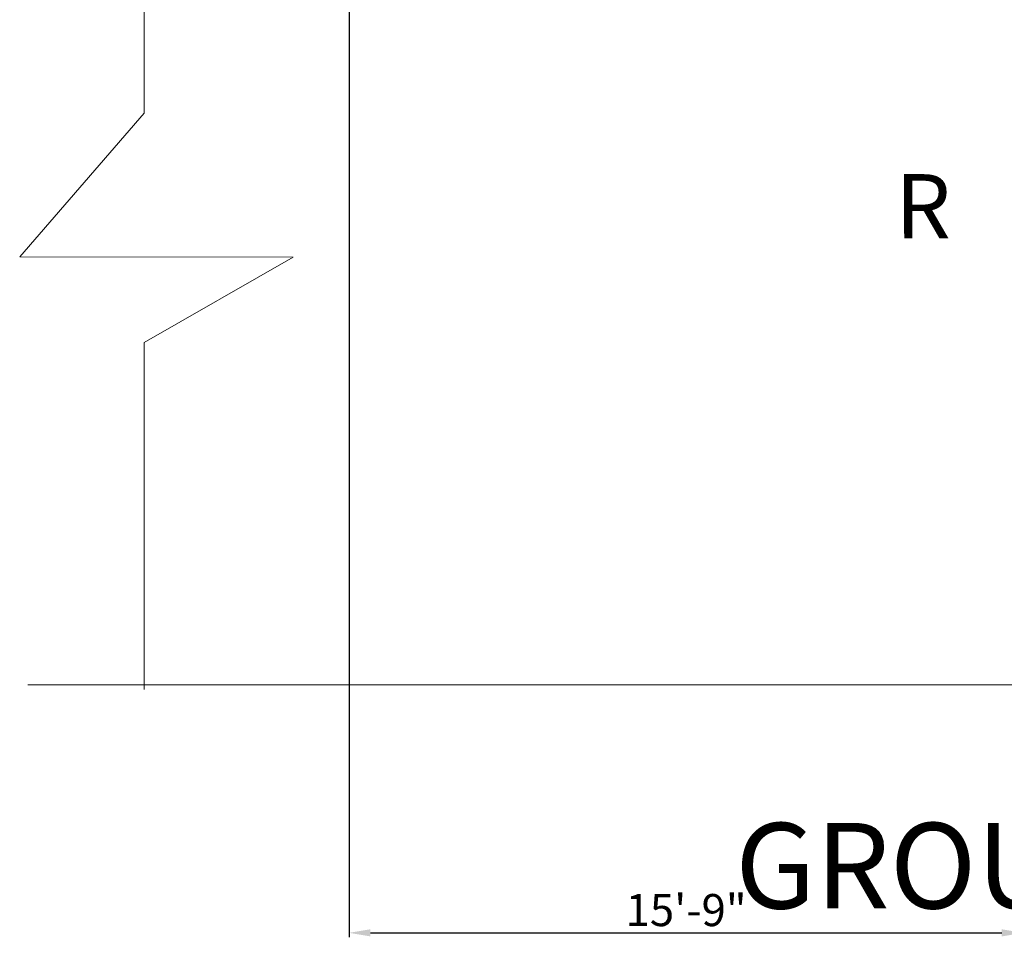
# Model space of a CAD drawing. Units: millimetres. Extents: x 595116 to 630915, y 909473 to 920225.
# Tile 2 of 134: x 629224 to 629500, y 918831 to 919089. Entities that reach past the tile are written whole.
import ezdxf

# ---------------------------------------------------------------- set-up
doc = ezdxf.new("R2010")
doc.units = ezdxf.units.MM
for name, color, linetype, lineweight in [('A-ANNO-TITL', 7, 'Continuous', 35), ('C-ROAD', 30, 'Continuous', 18), ('Dimension', 3, 'Continuous', 18), ('Text', 7, 'Continuous', 18)]:
    doc.layers.add(name, color=color, linetype=linetype, lineweight=lineweight)
doc.styles.get("Standard").update_dxf_attribs({"font": 'arial.ttf'})
doc.dimstyles.new('ISO-25', dxfattribs={"dimtxt": 9, "dimasz": 6, "dimexe": 1.25, "dimexo": 0.625, "dimtad": 1, "dimlunit": 4, "dimtxsty": 'Standard', "dimcen": 2.5, "dimadec": 0, "dimazin": 0, "dimtfac": 1, "dimtmove": 0, "dimatfit": 3, "dimfxl": 1, "dimarcsym": 0})

# ---------------------------------------------------------------- blocks, each defined once
blk = doc.blocks.new('*D215')
at = {"layer": 'Defpoints', "color": 0, "transparency": 16777216}
for p in [(629316.04, 919411.83), (629505.04, 919411.83), (629505.04, 918832.38)]:
    blk.add_point(p, dxfattribs=at)
at = {"layer": 'Dimension', "color": 0, "lineweight": -2, "transparency": 16777216}
for p, q in [((629316.04, 919411.2), (629316.04, 918831.13)), ((629505.04, 919411.2), (629505.04, 918831.13)), ((629322.04, 918832.38), (629499.04, 918832.38))]:
    blk.add_line(p, q, dxfattribs=at)
at = {"layer": 'Dimension', "color": 0, "transparency": 16777216}
for points in [[(629322.04, 918833.38), (629322.04, 918831.38), (629316.04, 918832.38)], [(629499.04, 918833.38), (629499.04, 918831.38), (629505.04, 918832.38)]]:
    blk.add_solid(points, dxfattribs=at)
at = {"layer": 'Dimension', "color": 0, "transparency": 16777216, "insert": (629410.54, 918837.6), "char_height": 9, "attachment_point": 5}
blk.add_mtext('15\'-9"', dxfattribs=at)

msp = doc.modelspace()

# ---------------------------------------------------------------- linework, layer by layer
at = {"layer": 'C-ROAD'}
msp.add_line((629225.95, 918901.928), (629943.895, 918901.928), dxfattribs=at)
msp.add_lwpolyline([(629258.594, 919143.178), (629258.594, 919062.342), (629223.682, 919021.992), (629300.343, 919021.872), (629258.594, 918997.995), (629258.594, 918900.678)], dxfattribs=at)

# ---------------------------------------------------------------- texts
at = {"layer": 'A-ANNO-TITL', "insert": (629372.977, 918863.187), "char_height": 24, "attachment_point": 1, "rotation": 0.01833}
msp.add_mtext_dynamic_manual_height_columns('{       GROUND FLOOR}', width=350.55928, gutter_width=12.5, heights=[0], dxfattribs=at)
at = {"layer": 'Text', "insert": (629469.211, 919045.194), "char_height": 18, "attachment_point": 1, "rotation": 0.01833}
msp.add_mtext_dynamic_manual_height_columns('{R    O   A   D}', width=269.48254, gutter_width=12.5, heights=[0], dxfattribs=at)

# ---------------------------------------------------------------- dimensions: what is measured, and where the dimension line sits
at = {"layer": 'Dimension'}
dim = msp.add_linear_dim(base=(629505.041, 918832.378), p1=(629316.041, 919411.828), p2=(629505.041, 919411.828), dimstyle='ISO-25', override={"dimdec": 1, "dimlfac": 1, "dimrnd": 0, "dimzin": 1, "dimdsep": 46, "dimlunit": 4, "dimfrac": 2}, dxfattribs=at)
dim.commit()
dim.dimension.update_dxf_attribs({"geometry": '*D215', "text_midpoint": (629410.541, 918837.598)})

doc.saveas('drawing.dxf')
